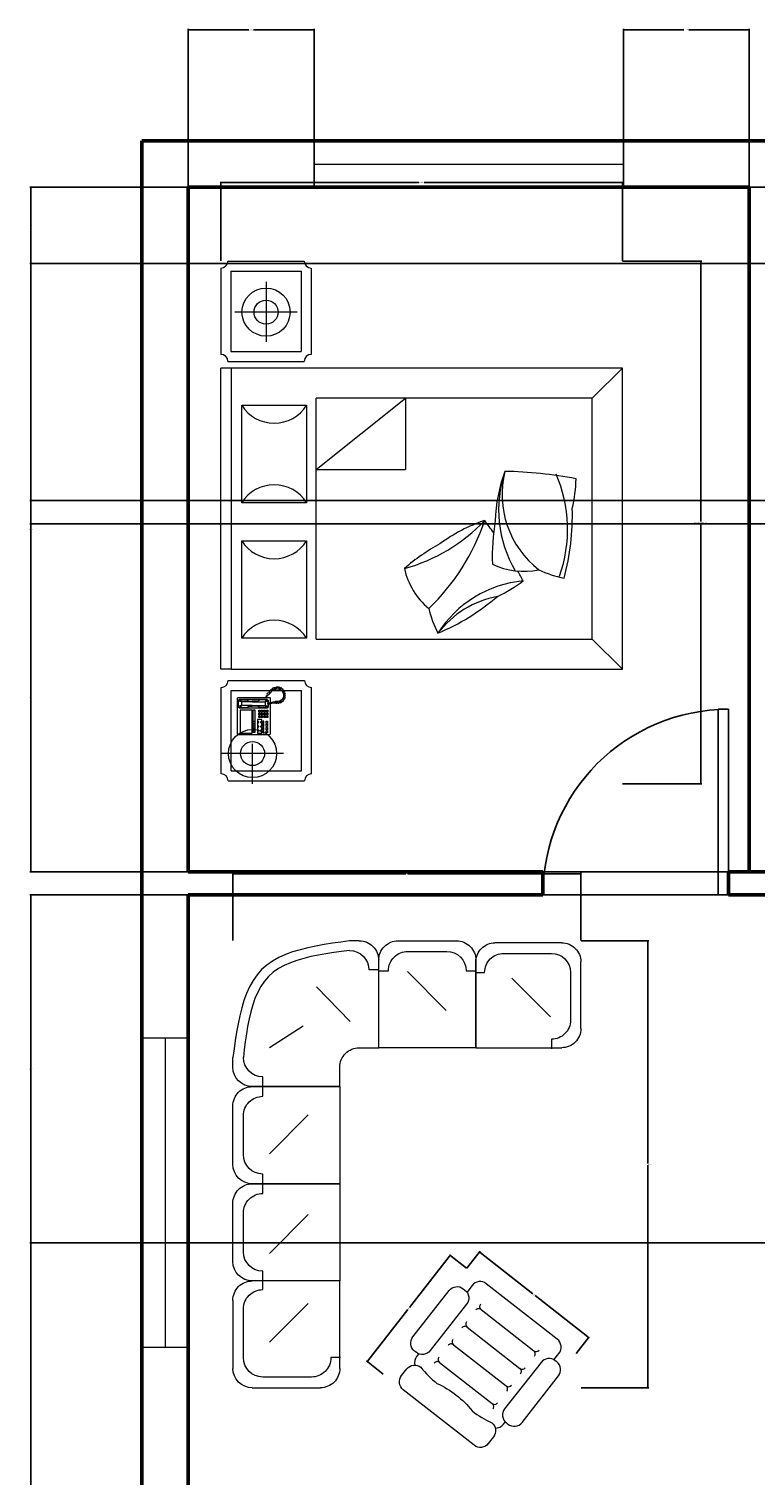
# Model space of a CAD drawing. Units: inches. Extents: x -108 to 1456, y -102 to 617.
# Tile 4 of 8: x 204 to 345, y 337 to 617. Entities that reach past the tile are written whole.
import ezdxf

# ---------------------------------------------------------------- set-up
doc = ezdxf.new("R2010")
doc.units = ezdxf.units.IN
for name, color, linetype, lineweight in [('A-ANNO-DIMS', 2, 'Continuous', 18), ('A-DOOR', 3, 'Continuous', 25), ('A-FURN', 8, 'Continuous', 18), ('A-GLAZ', 4, 'Continuous', 18), ('A-WALL', 7, 'Continuous', 50)]:
    doc.layers.add(name, color=color, linetype=linetype, lineweight=lineweight)
doc.styles.get("Standard").update_dxf_attribs({"font": 'arial.ttf'})
doc.dimstyles.get("Standard").update_dxf_attribs({"dimtxt": 0.18, "dimasz": 0.18, "dimexe": 0.18, "dimexo": 0.0625, "dimgap": 0.09, "dimtad": 0, "dimtih": 1, "dimtoh": 1, "dimdec": 4, "dimzin": 0, "dimdsep": 46, "dimtxsty": 'Standard', "dimcen": 0.09, "dimadec": 0, "dimazin": 0, "dimtfac": 1, "dimtdec": 4, "dimtofl": 0, "dimtmove": 0, "dimatfit": 3, "dimfxl": 1, "dimtolj": 1, "dimtzin": 0, "dimarcsym": 0})

# ---------------------------------------------------------------- blocks, each defined once
blk = doc.blocks.new('A$C50B66110')
for p, q in [((0.0153, 1.9631), (0.0153, 1.5831)), ((0.0503, 1.9981), (0.4803, 1.9981)), ((0.0653, 1.9481), (0.0653, 1.5981)), ((0.0653, 1.9481), (0.4653, 1.9481)), ((0.1513, 1.6871), (0.1513, 1.9967)), ((0.4653, 1.9481), (0.4653, 1.5981)), ((0.5153, 1.9631), (0.5153, 1.5831)), ((0.5716, 1.9488), (0.5716, 2)), ((0.5716, 2), (2.0719, 2)), ((2.0719, 1.9488), (0.5716, 1.9488)), ((0.5716, 1.9488), (0.5716, 0)), ((2.0719, 1.9488), (2.0719, 2)), ((2.0719, 0), (2.0719, 1.9488)), ((2.1051, 1.9643), (2.1051, 1.5843)), ((2.5701, 1.9993), (2.1401, 1.9993)), ((2.1551, 1.9493), (2.1551, 1.5993)), ((2.5551, 1.9493), (2.1551, 1.9493)), ((2.5551, 1.9493), (2.5551, 1.5993)), ((2.6051, 1.9643), (2.6051, 1.5843)), ((0.7257, 1.5725), (0.7257, 1.8954)), ((0.7257, 1.8954), (1.2113, 1.8954)), ((1.2113, 1.8954), (1.2113, 1.5725)), ((1.4007, 1.5725), (1.4007, 1.8954)), ((1.4007, 1.8954), (1.8863, 1.8954)), ((1.8863, 1.8954), (1.8863, 1.5725)), ((2.3505, 1.62), (2.3505, 1.9295)), ((0, 1.8416), (0.2001, 1.8416)), ((2.5018, 1.7744), (2.2017, 1.7744)), ((0.0653, 1.5981), (0.4653, 1.5981)), ((2.5551, 1.5993), (2.1551, 1.5993)), ((0.0503, 1.5481), (0.4803, 1.5481)), ((1.2113, 1.5725), (0.7257, 1.5725)), ((1.8863, 1.5725), (1.4007, 1.5725)), ((1.5665, 1.5254), (1.5665, 1.0802)), ((1.5665, 1.5254), (1.9219, 1.0802)), ((2.5701, 1.5493), (2.1401, 1.5493)), ((1.9219, 1.0802), (1.5665, 1.0802)), ((0.5716, 0), (0.7216, 0.15)), ((2.0719, 0), (1.9219, 0.15)), ((0.5716, 0), (2.0719, 0))]:
    blk.add_line(p, q)
at = {"linetype": 'ByBlock'}
for p, q in [((0.2481, 1.9162), (0.2458, 1.9139)), ((0.2458, 1.9139), (0.2458, 1.7562)), ((0.2481, 1.9162), (0.4287, 1.9162)), ((0.2526, 1.9036), (0.2526, 1.8431)), ((0.3669, 1.9036), (0.2526, 1.9036)), ((0.3669, 1.8431), (0.3669, 1.9036)), ((0.3772, 1.9071), (0.3818, 1.9128)), ((0.3772, 1.7688), (0.3772, 1.9071)), ((0.3818, 1.9094), (0.3807, 1.9048)), ((0.3807, 1.9048), (0.3807, 1.8739)), ((0.3807, 1.9048), (0.3909, 1.8945)), ((0.3807, 1.8739), (0.3829, 1.8682)), ((0.3818, 1.9128), (0.4161, 1.9128)), ((0.3864, 1.9116), (0.3818, 1.9094)), ((0.3921, 1.8968), (0.3864, 1.9116)), ((0.3864, 1.9116), (0.4138, 1.9116)), ((0.3909, 1.8945), (0.3921, 1.8968)), ((0.3909, 1.8431), (0.3909, 1.8945)), ((0.4081, 1.8968), (0.3921, 1.8968)), ((0.4081, 1.8968), (0.4138, 1.9116)), ((0.4092, 1.8945), (0.4081, 1.8968)), ((0.4195, 1.9048), (0.4092, 1.8945)), ((0.4092, 1.8431), (0.4092, 1.8945)), ((0.4138, 1.9116), (0.4184, 1.9094)), ((0.4161, 1.9128), (0.4218, 1.9071)), ((0.4195, 1.8739), (0.4172, 1.8682)), ((0.4184, 1.9094), (0.4195, 1.9048)), ((0.4195, 1.9048), (0.4195, 1.8739)), ((0.4218, 1.9071), (0.4218, 1.7699)), ((0.4287, 1.9162), (0.4309, 1.9139)), ((0.4309, 1.9139), (0.4309, 1.7562)), ((0.2526, 1.8431), (0.3669, 1.8431)), ((0.3201, 1.8168), (0.2526, 1.8168)), ((0.2526, 1.8168), (0.2526, 1.7962)), ((0.2572, 1.8408), (0.2572, 1.8294)), ((0.3669, 1.8408), (0.2572, 1.8408)), ((0.2572, 1.8294), (0.3669, 1.8294)), ((0.2675, 1.8145), (0.2641, 1.8145)), ((0.2641, 1.8145), (0.2641, 1.8111)), ((0.2641, 1.8111), (0.2675, 1.8111)), ((0.2641, 1.8019), (0.2641, 1.7985)), ((0.2675, 1.8019), (0.2641, 1.8019)), ((0.2664, 1.8408), (0.2664, 1.8294)), ((0.2675, 1.8111), (0.2675, 1.8145)), ((0.2675, 1.7985), (0.2675, 1.8019)), ((0.2755, 1.8408), (0.2755, 1.8294)), ((0.2846, 1.8408), (0.2846, 1.8294)), ((0.2846, 1.8145), (0.2846, 1.8111)), ((0.2881, 1.8145), (0.2846, 1.8145)), ((0.2846, 1.8111), (0.2881, 1.8111)), ((0.2846, 1.8019), (0.2846, 1.7985)), ((0.2881, 1.8019), (0.2846, 1.8019)), ((0.2881, 1.8111), (0.2881, 1.8145)), ((0.2881, 1.7985), (0.2881, 1.8019)), ((0.2938, 1.8408), (0.2938, 1.8294)), ((0.3029, 1.8408), (0.3029, 1.8294)), ((0.3052, 1.8145), (0.3052, 1.8111)), ((0.3086, 1.8145), (0.3052, 1.8145)), ((0.3052, 1.8111), (0.3086, 1.8111)), ((0.3052, 1.8019), (0.3052, 1.7985)), ((0.3086, 1.8019), (0.3052, 1.8019)), ((0.3086, 1.8111), (0.3086, 1.8145)), ((0.3086, 1.7985), (0.3086, 1.8019)), ((0.3121, 1.8408), (0.3121, 1.8294)), ((0.3201, 1.7962), (0.3201, 1.8168)), ((0.3304, 1.8111), (0.3395, 1.8111)), ((0.3304, 1.8042), (0.3304, 1.8111)), ((0.3395, 1.8042), (0.3304, 1.8042)), ((0.3395, 1.8111), (0.3395, 1.8042)), ((0.3441, 1.8042), (0.3441, 1.8111)), ((0.3441, 1.8111), (0.3532, 1.8111)), ((0.3532, 1.8042), (0.3441, 1.8042)), ((0.3532, 1.8111), (0.3532, 1.8042)), ((0.3578, 1.8111), (0.3669, 1.8111)), ((0.3578, 1.8042), (0.3578, 1.8111)), ((0.3669, 1.8042), (0.3578, 1.8042)), ((0.3669, 1.8294), (0.3669, 1.8408)), ((0.3669, 1.8111), (0.3669, 1.8042)), ((0.3807, 1.8019), (0.3829, 1.8076)), ((0.3807, 1.7711), (0.3807, 1.8019)), ((0.3829, 1.8682), (0.3864, 1.8625)), ((0.3829, 1.8076), (0.3864, 1.8134)), ((0.3864, 1.8625), (0.3875, 1.8545)), ((0.3864, 1.8134), (0.3875, 1.8214)), ((0.3875, 1.8545), (0.3875, 1.8431)), ((0.3875, 1.8214), (0.3875, 1.8431)), ((0.3909, 1.8431), (0.3909, 1.7813)), ((0.4092, 1.8431), (0.4092, 1.7813)), ((0.4138, 1.8625), (0.4127, 1.8545)), ((0.4127, 1.8545), (0.4127, 1.8431)), ((0.4127, 1.8214), (0.4127, 1.8431)), ((0.4138, 1.8134), (0.4127, 1.8214)), ((0.4172, 1.8682), (0.4138, 1.8625)), ((0.4172, 1.8076), (0.4138, 1.8134)), ((0.4195, 1.8019), (0.4172, 1.8076)), ((0.4195, 1.7711), (0.4195, 1.8019)), ((0.2458, 1.7562), (0.2481, 1.7539)), ((0.4, 1.7539), (0.2481, 1.7539)), ((0.2526, 1.7962), (0.3201, 1.7962)), ((0.2652, 1.7905), (0.2538, 1.7905)), ((0.2538, 1.7905), (0.2538, 1.7859)), ((0.2538, 1.7859), (0.2652, 1.7859)), ((0.2538, 1.7665), (0.2538, 1.7733)), ((0.2538, 1.7733), (0.2652, 1.7733)), ((0.2652, 1.7665), (0.2538, 1.7665)), ((0.2641, 1.7985), (0.2675, 1.7985)), ((0.2652, 1.7859), (0.2652, 1.7905)), ((0.2652, 1.7733), (0.2652, 1.7665)), ((0.2812, 1.7905), (0.2698, 1.7905)), ((0.2698, 1.7905), (0.2698, 1.7859)), ((0.2698, 1.7859), (0.2812, 1.7859)), ((0.2698, 1.7665), (0.2698, 1.7733)), ((0.2698, 1.7733), (0.2812, 1.7733)), ((0.2812, 1.7665), (0.2698, 1.7665)), ((0.2812, 1.7859), (0.2812, 1.7905)), ((0.2812, 1.7733), (0.2812, 1.7665)), ((0.2846, 1.7985), (0.2881, 1.7985)), ((0.2972, 1.7905), (0.2858, 1.7905)), ((0.2858, 1.7905), (0.2858, 1.7859)), ((0.2858, 1.7859), (0.2972, 1.7859)), ((0.2858, 1.7665), (0.2858, 1.7733)), ((0.2858, 1.7733), (0.2972, 1.7733)), ((0.2972, 1.7665), (0.2858, 1.7665)), ((0.2972, 1.7859), (0.2972, 1.7905)), ((0.2972, 1.7733), (0.2972, 1.7665)), ((0.3018, 1.7905), (0.3018, 1.7859)), ((0.3132, 1.7905), (0.3018, 1.7905)), ((0.3018, 1.7859), (0.3132, 1.7859)), ((0.3018, 1.7733), (0.3132, 1.7733)), ((0.3018, 1.7665), (0.3018, 1.7733)), ((0.3132, 1.7665), (0.3018, 1.7665)), ((0.3052, 1.7985), (0.3086, 1.7985)), ((0.3132, 1.7859), (0.3132, 1.7905)), ((0.3132, 1.7733), (0.3132, 1.7665)), ((0.3304, 1.7985), (0.3395, 1.7985)), ((0.3304, 1.7916), (0.3304, 1.7985)), ((0.3395, 1.7916), (0.3304, 1.7916)), ((0.3304, 1.7779), (0.3304, 1.7848)), ((0.3304, 1.7848), (0.3395, 1.7848)), ((0.3395, 1.7779), (0.3304, 1.7779)), ((0.3304, 1.7722), (0.3395, 1.7722)), ((0.3304, 1.7653), (0.3304, 1.7722)), ((0.3395, 1.7653), (0.3304, 1.7653)), ((0.3395, 1.7985), (0.3395, 1.7916)), ((0.3395, 1.7848), (0.3395, 1.7779)), ((0.3395, 1.7722), (0.3395, 1.7653)), ((0.3441, 1.7985), (0.3532, 1.7985)), ((0.3441, 1.7916), (0.3441, 1.7985)), ((0.3532, 1.7916), (0.3441, 1.7916)), ((0.3441, 1.7779), (0.3441, 1.7848)), ((0.3441, 1.7848), (0.3532, 1.7848)), ((0.3532, 1.7779), (0.3441, 1.7779)), ((0.3441, 1.7722), (0.3532, 1.7722)), ((0.3441, 1.7653), (0.3441, 1.7722)), ((0.3532, 1.7653), (0.3441, 1.7653)), ((0.3532, 1.7985), (0.3532, 1.7916)), ((0.3532, 1.7848), (0.3532, 1.7779)), ((0.3532, 1.7722), (0.3532, 1.7653)), ((0.3578, 1.7985), (0.3669, 1.7985)), ((0.3578, 1.7916), (0.3578, 1.7985)), ((0.3669, 1.7916), (0.3578, 1.7916)), ((0.3578, 1.7791), (0.3578, 1.7859)), ((0.3578, 1.7859), (0.3669, 1.7859)), ((0.3669, 1.7791), (0.3578, 1.7791)), ((0.3578, 1.7653), (0.3578, 1.7722)), ((0.3578, 1.7722), (0.3669, 1.7722)), ((0.3669, 1.7653), (0.3578, 1.7653)), ((0.3669, 1.7985), (0.3669, 1.7916)), ((0.3669, 1.7859), (0.3669, 1.7791)), ((0.3669, 1.7722), (0.3669, 1.7653)), ((0.3829, 1.7631), (0.3772, 1.7688)), ((0.3807, 1.7711), (0.3909, 1.7813)), ((0.3818, 1.7665), (0.3807, 1.7711)), ((0.3864, 1.7642), (0.3818, 1.7665)), ((0.399, 1.7631), (0.3829, 1.7631)), ((0.3921, 1.7791), (0.3864, 1.7642)), ((0.3864, 1.7642), (0.399, 1.7642)), ((0.3909, 1.7813), (0.3921, 1.7791)), ((0.4081, 1.7791), (0.3921, 1.7791)), ((0.4024, 1.7676), (0.3989, 1.7676)), ((0.3989, 1.7676), (0.3991, 1.7578)), ((0.3991, 1.7578), (0.4019, 1.7462)), ((0.4019, 1.7462), (0.4047, 1.7353)), ((0.403, 1.7585), (0.4024, 1.7676)), ((0.4026, 1.7642), (0.4138, 1.7642)), ((0.4161, 1.7631), (0.4027, 1.7631)), ((0.4047, 1.7511), (0.403, 1.7585)), ((0.4287, 1.7539), (0.404, 1.7539)), ((0.4047, 1.7353), (0.4044, 1.7293)), ((0.4044, 1.7293), (0.4051, 1.7279)), ((0.4074, 1.7402), (0.4047, 1.7511)), ((0.4081, 1.7346), (0.4074, 1.7402)), ((0.4079, 1.7286), (0.4081, 1.7346)), ((0.4092, 1.7813), (0.4081, 1.7791)), ((0.4081, 1.7791), (0.4138, 1.7642)), ((0.4195, 1.7711), (0.4092, 1.7813)), ((0.4138, 1.7642), (0.4184, 1.7665)), ((0.4218, 1.7699), (0.4161, 1.7631)), ((0.4184, 1.7665), (0.4195, 1.7711)), ((0.4309, 1.7562), (0.4287, 1.7539)), ((0.4378, 1.7742), (0.4309, 1.7768)), ((0.4309, 1.7722), (0.436, 1.7708)), ((0.436, 1.7708), (0.4406, 1.7672)), ((0.441, 1.771), (0.4378, 1.7742)), ((0.4406, 1.7672), (0.4418, 1.7656)), ((0.4434, 1.7688), (0.441, 1.771)), ((0.4443, 1.7658), (0.4418, 1.7633)), ((0.4418, 1.7656), (0.4443, 1.7658)), ((0.4418, 1.7633), (0.4511, 1.7551)), ((0.4477, 1.7704), (0.4434, 1.7688)), ((0.4497, 1.7684), (0.4477, 1.7704)), ((0.4481, 1.765), (0.4497, 1.7684)), ((0.4509, 1.7672), (0.4481, 1.765)), ((0.4539, 1.764), (0.4509, 1.7672)), ((0.4511, 1.7551), (0.4662, 1.7422)), ((0.4515, 1.7573), (0.4539, 1.764)), ((0.4577, 1.7605), (0.4515, 1.7573)), ((0.463, 1.7555), (0.4577, 1.7605)), ((0.4618, 1.7482), (0.463, 1.7555)), ((0.467, 1.7515), (0.4618, 1.7482)), ((0.4664, 1.7418), (0.4741, 1.72)), ((0.4714, 1.7468), (0.467, 1.7515)), ((0.4696, 1.7418), (0.4714, 1.7468)), ((0.4766, 1.7425), (0.4697, 1.7418)), ((0.472, 1.733), (0.4787, 1.7356)), ((0.4794, 1.7332), (0.472, 1.733)), ((0.4787, 1.7356), (0.4766, 1.7425)), ((0.481, 1.7279), (0.4794, 1.7332)), ((0.4026, 1.7254), (0.4021, 1.7198)), ((0.4021, 1.7198), (0.4088, 1.7187)), ((0.4088, 1.7187), (0.4023, 1.7147)), ((0.4023, 1.7147), (0.4028, 1.7085)), ((0.4051, 1.7279), (0.4026, 1.7254)), ((0.4028, 1.7085), (0.4102, 1.7078)), ((0.4102, 1.7078), (0.4037, 1.7027)), ((0.4037, 1.7027), (0.4067, 1.6974)), ((0.4067, 1.6974), (0.4137, 1.6988)), ((0.4121, 1.7256), (0.4079, 1.7286)), ((0.4137, 1.6988), (0.4104, 1.6923)), ((0.4104, 1.6923), (0.4139, 1.6881)), ((0.4111, 1.7203), (0.4121, 1.7256)), ((0.4123, 1.7057), (0.4111, 1.7203)), ((0.4211, 1.6946), (0.4123, 1.7057)), ((0.4139, 1.6881), (0.4192, 1.692)), ((0.4192, 1.692), (0.4183, 1.6858)), ((0.4183, 1.6858), (0.4227, 1.683)), ((0.4333, 1.6881), (0.4211, 1.6946)), ((0.4227, 1.683), (0.4283, 1.6876)), ((0.4283, 1.6876), (0.4276, 1.68)), ((0.4276, 1.68), (0.4324, 1.6786)), ((0.4324, 1.6786), (0.4354, 1.6849)), ((0.4472, 1.6869), (0.4333, 1.6881)), ((0.4354, 1.6849), (0.4382, 1.6786)), ((0.4382, 1.6786), (0.4421, 1.6782)), ((0.4421, 1.6782), (0.4437, 1.6849)), ((0.4437, 1.6849), (0.4463, 1.6775)), ((0.4463, 1.6775), (0.4507, 1.6786)), ((0.4606, 1.6927), (0.4472, 1.6869)), ((0.4507, 1.6786), (0.4509, 1.6849)), ((0.4509, 1.6849), (0.4562, 1.6802)), ((0.4562, 1.6802), (0.4599, 1.6821)), ((0.4592, 1.689), (0.4641, 1.683)), ((0.4599, 1.6821), (0.4592, 1.689)), ((0.4708, 1.7027), (0.4606, 1.6927)), ((0.4641, 1.683), (0.4678, 1.6863)), ((0.465, 1.6925), (0.4715, 1.6897)), ((0.4678, 1.6863), (0.465, 1.6925)), ((0.4741, 1.72), (0.4708, 1.7027)), ((0.4745, 1.6925), (0.4713, 1.6988)), ((0.4713, 1.6988), (0.478, 1.6967)), ((0.4715, 1.6897), (0.4745, 1.6925)), ((0.4743, 1.7075), (0.4815, 1.7073)), ((0.4798, 1.7013), (0.4743, 1.7075)), ((0.4761, 1.7233), (0.481, 1.7279)), ((0.4824, 1.7233), (0.4761, 1.7233)), ((0.4764, 1.7154), (0.4835, 1.7175)), ((0.4824, 1.7119), (0.4764, 1.7154)), ((0.478, 1.6967), (0.4798, 1.7013)), ((0.4815, 1.7073), (0.4824, 1.7119)), ((0.4835, 1.7175), (0.4824, 1.7233)), ((0.7216, 1.5254), (1.9219, 1.5254)), ((0.7216, 1.5254), (0.7216, 0.15)), ((1.9219, 0.15), (1.9219, 1.5254)), ((0.7216, 0.15), (1.9219, 0.15))]:
    blk.add_line(p, q, dxfattribs=at)
for centre, radius in [((0.1513, 1.8416), 0.12), ((0.1513, 1.8416), 0.06), ((2.3505, 1.7744), 0.12), ((2.3505, 1.7744), 0.06)]:
    blk.add_circle(centre, radius)
for centre, radius, start, end in [((0.0153, 1.9981), 0.035, 270, 0), ((0.5153, 1.9981), 0.035, 180, 270), ((2.1051, 1.9993), 0.035, 270, 0), ((2.6051, 1.9993), 0.035, 180, 270), ((0.6244, 1.734), 0.1906, 302.12017, 57.87983), ((1.3126, 1.734), 0.1906, 122.12017, 237.87983), ((1.2994, 1.734), 0.1906, 302.12017, 57.87983), ((1.9876, 1.734), 0.1906, 122.12017, 237.87983), ((0.0153, 1.5481), 0.035, 0, 90), ((0.5153, 1.5481), 0.035, 90, 180), ((2.1051, 1.5493), 0.035, 0, 90), ((2.6051, 1.5493), 0.035, 90, 180), ((1.1502, 0.7366), 0.3575, 102.47819, 140.46254), ((0.328, 0.4368), 0.9879, 28.49711, 41.05657), ((1.9117, 1.3157), 0.8697, 195.33601, 226.41927), ((0.9996, 0.4307), 0.548, 103.20343, 117.03623), ((1.656, 1.7093), 1.0798, 223.63057, 251.4288), ((0.4482, 0.4408), 0.5655, 5.33912, 57.68949), ((1.8226, 1.3753), 1.1652, 203.06416, 220.32086), ((0.4548, 0.5307), 0.4879, 10.69865, 52.68638), ((0.5648, 0.4378), 0.7874, 18.35266, 36.68512), ((-0.0179, 2.4352), 2.1977, 305.29657, 307.24182), ((1.5981, 0.9345), 0.734, 205.25901, 216.93514), ((1.4166, 0.4903), 0.3575, 154.0418, 192.02615), ((1.3672, 0.0075), 0.6085, 71.81005, 120.13512), ((1.4431, 0.1219), 0.4774, 76.18494, 142.00166), ((1.1403, -0.3401), 0.9879, 80.06073, 92.62018), ((1.2867, -0.154), 0.7874, 69.91627, 88.24873), ((-0.6401, 0.6314), 2.1977, 349.48843, 358.80544), ((-0.0179, 2.4352), 2.1977, 297.92482, 299.3793), ((1.5626, 0.1822), 0.548, 154.76704, 168.59984), ((1.3343, 1.4141), 1.1652, 254.62778, 271.88448), ((1.2678, 0.9611), 0.6885, 250.29361, 293.6414), ((1.5399, 0.9642), 0.734, 256.82263, 268.49876)]:
    blk.add_arc(centre, radius, start, end)
blk = doc.blocks.new('A$C4B324E0D')
for points in [[(-0.4032, -0.0374), (-0.3959, 0.0153), (-0.3883, 0.0678), (-0.3801, 0.1195), (-0.3709, 0.1704), (-0.3605, 0.22), (-0.3485, 0.2679), (-0.3346, 0.314), (-0.3185, 0.3579), (-0.2998, 0.3993), (-0.2783, 0.4378), (-0.2537, 0.4731), (-0.2255, 0.5049), (-0.1936, 0.5331), (-0.1583, 0.5578), (-0.1198, 0.5793), (-0.0785, 0.5979), (-0.0346, 0.614), (0.0115, 0.628), (0.0595, 0.64), (0.1091, 0.6504), (0.1599, 0.6595), (0.2117, 0.6678), (0.2641, 0.6753), (0.3168, 0.6826)], [(0.3768, 0.6826), (0.3168, 0.6826)], [(0.9768, 0.6826), (0.6168, 0.6826)], [(1.5769, 0.6826), (1.2168, 0.6826)], [(1.8168, 0.6826), (2.2368, 0.6826)], [(-0.3432, -0.0374), (-0.3369, 0.0114), (-0.3303, 0.0599), (-0.3232, 0.1078), (-0.3151, 0.1548), (-0.3059, 0.2006), (-0.2951, 0.2449), (-0.2826, 0.2874), (-0.2681, 0.3278), (-0.2511, 0.3658), (-0.2315, 0.4011), (-0.2089, 0.4335), (-0.1831, 0.4625), (-0.1538, 0.488), (-0.1214, 0.5102), (-0.086, 0.5294), (-0.0479, 0.546), (-0.0075, 0.5602), (0.035, 0.5722), (0.0793, 0.5825), (0.125, 0.5914), (0.172, 0.599), (0.2198, 0.6057), (0.2682, 0.6119), (0.3168, 0.6177)], [(0.3168, 0.6177), (0.3168, 0.6177)], [(0.4968, 0.0226), (0.4968, 0.5626)], [(0.4968, 0.5626), (0.4968, 0.0226), (1.0968, 0.0226)], [(0.9168, 0.6177), (0.6768, 0.6177)], [(1.0968, 0.5626), (1.0968, 0.0226), (1.6968, 0.0226)], [(1.0968, 0.0226), (1.0968, 0.5626)], [(1.5168, 0.6177), (1.2768, 0.6177)], [(1.6968, 0.0226), (1.6968, 0.5626)], [(2.2368, 0.0226), (1.6968, 0.0226), (1.6968, 0.5626)], [(2.1704, 0.6177), (1.8704, 0.6177)], [(2.3569, 0.5626), (2.3569, 0.1426)], [(0.255, 0.4573), (0.1211, 0.2495)], [(0.4968, 0.4977), (0.4368, 0.4977), (0.4368, 0.4977)], [(0.5569, 0.4977), (0.5569, 0.4977), (0.4968, 0.4977)], [(0.9111, 0.4573), (0.6711, 0.2173)], [(1.0968, 0.4977), (1.0368, 0.4977), (1.0368, 0.4977)], [(1.1569, 0.4977), (1.1569, 0.4977), (1.0968, 0.4977)], [(1.527, 0.4573), (1.287, 0.2173)], [(1.6969, 0.4977), (1.6368, 0.4977), (1.6368, 0.4977)], [(1.7504, 0.4977), (1.7504, 0.4977), (1.6904, 0.4977)], [(2.0759, 0.4573), (1.8359, 0.2173)], [(2.2904, 0.1977), (2.2904, 0.4977)], [(-0.1199, 0.1664), (0.0943, -0.0414)], [(0.4968, 0.0226), (0.3768, 0.0226)], [(2.1704, 0.0177), (2.1704, 0.0777), (2.1704, 0.0777)], [(-0.4032, -0.0974), (-0.4032, -0.0374)], [(-0.3432, -0.0374), (-0.3432, -0.0374)], [(-0.2232, -0.2174), (-0.2232, -0.1574), (-0.2232, -0.1574)], [(0.2568, -0.0974), (0.2568, -0.2174)], [(-0.2832, -0.8174), (0.2568, -0.8174), (0.2568, -0.2174)], [(0.2568, -0.2174), (-0.2832, -0.2174)], [(0.2568, -0.2174), (-0.2832, -0.2174)], [(-0.2183, -0.2174), (-0.2183, -0.2774), (-0.2183, -0.2774)], [(-0.4032, -0.3374), (-0.4032, -0.6974)], [(-0.3383, -0.3974), (-0.3383, -0.6374)], [(-0.2136, -0.3946), (0.0264, -0.6346)], [(-0.2183, -0.7574), (-0.2183, -0.7574), (-0.2183, -0.8174)], [(0.2568, -0.8174), (-0.2832, -0.8174)], [(-0.2732, -0.8174), (0.2568, -0.8174), (0.2568, -1.3475)], [(-0.208, -0.8126), (-0.208, -0.8715), (-0.208, -0.8715)], [(0.2568, -0.8174), (0.2568, -1.3475)], [(-0.391, -1.3475), (-0.391, -0.9352)], [(-0.3258, -0.9893), (-0.3258, -1.2838)], [(-0.1734, -1.0387), (0.0666, -1.2787)], [(0.2043, -1.2838), (0.2043, -1.2838), (0.2632, -1.2838)], [(-0.208, -1.4016), (0.0865, -1.4016)], [(0.1391, -1.4653), (-0.2732, -1.4653)]]:
    blk.add_lwpolyline(points)
for centre, radius, start, end in [((0.3768, 0.5626), 0.12, 0, 90), ((0.6168, 0.5626), 0.12, 90, 180), ((0.9768, 0.5626), 0.12, 0, 90), ((1.2168, 0.5626), 0.12, 90, 180), ((1.5769, 0.5626), 0.12, 0, 90), ((1.8168, 0.5626), 0.12, 90, 180), ((2.2368, 0.5626), 0.12, 0, 90), ((0.3168, 0.4977), 0.12, 0, 90), ((0.6768, 0.4977), 0.12, 90, 180), ((0.9168, 0.4977), 0.12, 0, 90), ((1.2768, 0.4977), 0.12, 90, 180), ((1.5168, 0.4977), 0.12, 0, 90), ((1.8704, 0.4977), 0.12, 90, 180), ((2.1704, 0.4977), 0.12, 0, 90), ((2.1704, 0.1977), 0.12, 270, 0), ((2.2368, 0.1426), 0.12, 270, 0), ((0.3768, -0.0974), 0.12, 90, 180), ((-0.2232, -0.0374), 0.12, 180, 270), ((-0.2832, -0.0974), 0.12, 179.9997, 270), ((-0.2832, -0.3374), 0.12, 90, 180), ((-0.2183, -0.3974), 0.12, 90, 180), ((-0.2832, -0.6974), 0.12, 179.9997, 270), ((-0.2183, -0.6374), 0.12, 180, 270), ((-0.2732, -0.9352), 0.1178, 90, 180), ((-0.208, -0.9893), 0.1178, 90, 180), ((-0.208, -1.2838), 0.1178, 180, 270), ((0.0865, -1.2838), 0.1178, 270, 0), ((-0.2732, -1.3475), 0.1178, 179.9997, 270), ((0.1391, -1.3475), 0.1178, 270, 0)]:
    blk.add_arc(centre, radius, start, end)
blk = doc.blocks.new('A$C58C6152E')
at = {"xscale": 1.5, "yscale": 1.5, "zscale": 1.5, "rotation": 90}
blk.add_blockref('A$C4B324E0D', (1.024, 0.605), dxfattribs=at)
blk = doc.blocks.new('A$C15DC316E')
at = {"xscale": -1, "rotation": 270}
blk.add_blockref('A$C58C6152E', (0, 0), dxfattribs=at)
blk = doc.blocks.new('A$C31080000')
for p, q in [((364.2, 324.1), (125.4, 324.1)), ((364.2, 244.1), (125.4, 244.1)), ((364.2, 164.1), (125.4, 164.1)), ((364.2, 84.1), (125.4, 84.1)), ((442.3, 35.8), (442.3, 67.5))]:
    blk.add_line(p, q)
for points in [[(48.5, 445.3, -0.414214), (84.3, 481.1), (406.4, 481.1, -0.414214), (442.2, 445.3), (442.2, 415.1, -0.414214), (406.4, 379.4)], [(406.4, 379.4, 0.055299), (325.4, 388.9, -0.118462), (165.4, 388.9, 0.055299), (84.3, 379.4, -0.414214), (48.5, 415.1), (48.5, 445.3, -0.414214)], [(62.9, 386.5, 0.236068), (48.5, 357.9), (48.5, 347.9)], [(442.2, 345.6), (442.2, 357.9, 0.236068), (427.9, 386.5)], [(48.5, 65.5), (48.5, 35.8, 0.414214), (84.3, 0), (406.4, 0, 0.414214), (442.2, 35.8)]]:
    blk.add_lwpolyline(points, format="xyb")
for points in [[(78.9, 311.7, 0.414214), (43.1, 347.5), (35.8, 347.5, 0.414214), (0, 311.7), (0, 100.6, 0.414214), (35.8, 64.8), (43.1, 64.8, 0.414214), (78.9, 100.6)], [(416.7, 311.7, -0.414214), (452.5, 347.5), (459.8, 347.5, -0.414214), (495.6, 311.7), (495.6, 100.6, -0.414214), (459.8, 64.8), (452.5, 64.8, -0.414214), (416.7, 100.6)]]:
    blk.add_lwpolyline(points, format="xyb", close=True)
for centre, start, end in [((125.4, 337.6), 180, 270), ((125.4, 310.5), 90, 180), ((364.2, 337.6), 270, 0), ((364.2, 310.5), 0, 90), ((125.4, 257.6), 180, 270), ((125.4, 230.5), 90, 180), ((364.2, 257.6), 270, 0), ((364.2, 230.5), 0, 90), ((125.4, 177.6), 180, 270), ((125.4, 150.5), 90, 180), ((364.2, 177.6), 270, 0), ((364.2, 150.5), 0, 90), ((125.4, 97.6), 180, 270), ((125.4, 70.5), 90, 180), ((364.2, 97.6), 270, 0), ((364.2, 70.5), 0, 90)]:
    blk.add_arc(centre, 13.6, start, end)
blk = doc.blocks.new('DOOR-36-SWING')
for p, q in [((36, 36), (34, 36)), ((34, 36), (34, 0)), ((36, 36), (34, 36)), ((36, 0), (36, 36)), ((34, 0), (36, 0))]:
    blk.add_line(p, q)
blk.add_arc((36, 36), 36, 180, 270)
blk = doc.blocks.new('WIN-60-WALL-9')
for p, q in [((0, 0), (0, 9)), ((60, 0), (60, 9)), ((0, 4.5), (60, 4.5))]:
    blk.add_line(p, q)
blk = doc.blocks.new('*D20')
at = {"layer": 'A-ANNO-DIMS', "color": 0, "lineweight": -2, "transparency": 16777216}
for p, q in [((319.55, 572.46), (334.88, 572.46)), ((334.7, 572.28), (334.7, 521.94)), ((334.7, 471.23), (334.7, 521.57)), ((319.55, 471.05), (334.88, 471.05))]:
    blk.add_line(p, q, dxfattribs=at)
at = {"layer": 'A-ANNO-DIMS', "color": 0, "transparency": 16777216}
for points in [[(334.67, 572.28), (334.73, 572.28), (334.7, 572.46)], [(334.67, 471.23), (334.73, 471.23), (334.7, 471.05)]]:
    blk.add_solid(points, dxfattribs=at)
at = {"layer": 'Defpoints', "color": 0, "transparency": 16777216}
for p in [(319.49, 572.46), (334.7, 572.46), (319.49, 471.05)]:
    blk.add_point(p, dxfattribs=at)
at = {"layer": 'A-ANNO-DIMS', "color": 0, "transparency": 16777216, "insert": (334.7, 521.75), "char_height": 0.18, "attachment_point": 5}
blk.add_mtext('\\A1;BED GROUP 101 TYP.', dxfattribs=at)
blk = doc.blocks.new('*D21')
at = {"layer": 'A-ANNO-DIMS', "color": 0, "lineweight": -2, "transparency": 16777216}
for p, q in [((241.63, 572.52), (241.63, 587.85)), ((241.81, 587.67), (280.03, 587.67)), ((319.31, 587.67), (281.09, 587.67)), ((319.49, 572.52), (319.49, 587.85))]:
    blk.add_line(p, q, dxfattribs=at)
at = {"layer": 'A-ANNO-DIMS', "color": 0, "transparency": 16777216}
for points in [[(241.81, 587.7), (241.81, 587.64), (241.63, 587.67)], [(319.31, 587.7), (319.31, 587.64), (319.49, 587.67)]]:
    blk.add_solid(points, dxfattribs=at)
at = {"layer": 'Defpoints', "color": 0, "transparency": 16777216}
for p in [(241.63, 587.67), (241.63, 572.46), (319.49, 572.46)]:
    blk.add_point(p, dxfattribs=at)
at = {"layer": 'A-ANNO-DIMS', "color": 0, "transparency": 16777216, "insert": (280.56, 587.67), "char_height": 0.18, "attachment_point": 5}
blk.add_mtext('\\A1;78 TYP.', dxfattribs=at)
blk = doc.blocks.new('*D30')
at = {"layer": 'A-ANNO-DIMS', "color": 0, "lineweight": -2, "transparency": 16777216}
for p, q in [((311.51, 440.62), (324.63, 440.62)), ((324.45, 440.44), (324.45, 397.46)), ((324.45, 354.11), (324.45, 397.09)), ((311.51, 353.93), (324.63, 353.93))]:
    blk.add_line(p, q, dxfattribs=at)
at = {"layer": 'A-ANNO-DIMS', "color": 0, "transparency": 16777216}
for points in [[(324.42, 440.44), (324.48, 440.44), (324.45, 440.62)], [(324.42, 354.11), (324.48, 354.11), (324.45, 353.93)]]:
    blk.add_solid(points, dxfattribs=at)
at = {"layer": 'Defpoints', "color": 0, "transparency": 16777216}
for p in [(311.44, 440.62), (311.44, 353.93), (324.45, 353.93)]:
    blk.add_point(p, dxfattribs=at)
at = {"layer": 'A-ANNO-DIMS', "color": 0, "transparency": 16777216, "insert": (324.45, 397.27), "char_height": 0.18, "attachment_point": 5}
blk.add_mtext('\\A1;SECTIONAL 87', dxfattribs=at)
blk = doc.blocks.new('*D31')
at = {"layer": 'A-ANNO-DIMS', "color": 0, "lineweight": -2, "transparency": 16777216}
for p, q in [((243.98, 440.68), (243.98, 453.8)), ((244.16, 453.62), (277.49, 453.62)), ((311.26, 453.62), (277.93, 453.62)), ((311.44, 440.68), (311.44, 453.8))]:
    blk.add_line(p, q, dxfattribs=at)
at = {"layer": 'A-ANNO-DIMS', "color": 0, "transparency": 16777216}
for points in [[(244.16, 453.65), (244.16, 453.59), (243.98, 453.62)], [(311.26, 453.65), (311.26, 453.59), (311.44, 453.62)]]:
    blk.add_solid(points, dxfattribs=at)
at = {"layer": 'Defpoints', "color": 0, "transparency": 16777216}
for p in [(311.44, 453.62), (243.98, 440.62), (311.44, 440.62)]:
    blk.add_point(p, dxfattribs=at)
at = {"layer": 'A-ANNO-DIMS', "color": 0, "transparency": 16777216, "insert": (277.71, 453.62), "char_height": 0.18, "attachment_point": 5}
blk.add_mtext('\\A1;67', dxfattribs=at)
blk = doc.blocks.new('*D32')
at = {"layer": 'A-ANNO-DIMS', "color": 0, "lineweight": -2, "transparency": 16777216}
for p, q in [((289.34, 377.15), (291.9, 380.42)), ((291.93, 380.17), (302.14, 372.17)), ((312.83, 363.8), (302.61, 371.8)), ((310.52, 360.56), (313.08, 363.83))]:
    blk.add_line(p, q, dxfattribs=at)
at = {"layer": 'A-ANNO-DIMS', "color": 0, "transparency": 16777216}
for points in [[(291.95, 380.19), (291.91, 380.14), (291.79, 380.28)], [(312.84, 363.83), (312.81, 363.78), (312.97, 363.69)]]:
    blk.add_solid(points, dxfattribs=at)
at = {"layer": 'Defpoints', "color": 0, "transparency": 16777216}
for p in [(291.79, 380.28), (289.3, 377.1), (310.48, 360.51)]:
    blk.add_point(p, dxfattribs=at)
at = {"layer": 'A-ANNO-DIMS', "color": 0, "transparency": 16777216, "insert": (302.38, 371.98), "char_height": 0.18, "attachment_point": 5}
blk.add_mtext('\\A1;CHAIR 27', dxfattribs=at)
blk = doc.blocks.new('*D33')
at = {"layer": 'A-ANNO-DIMS', "color": 0, "lineweight": -2, "transparency": 16777216}
for p, q in [((286.01, 379.45), (278.21, 369.49)), ((289.25, 377.14), (285.98, 379.7)), ((270.13, 359.17), (277.93, 369.13)), ((273.15, 356.58), (269.88, 359.14))]:
    blk.add_line(p, q, dxfattribs=at)
at = {"layer": 'A-ANNO-DIMS', "color": 0, "transparency": 16777216}
for points in [[(285.99, 379.47), (286.03, 379.43), (286.12, 379.59)], [(270.1, 359.19), (270.15, 359.15), (270.02, 359.03)]]:
    blk.add_solid(points, dxfattribs=at)
at = {"layer": 'Defpoints', "color": 0, "transparency": 16777216}
for p in [(289.3, 377.1), (270.02, 359.03), (273.19, 356.54)]:
    blk.add_point(p, dxfattribs=at)
at = {"layer": 'A-ANNO-DIMS', "color": 0, "transparency": 16777216, "insert": (278.07, 369.31), "char_height": 0.18, "attachment_point": 5}
blk.add_mtext('\\A1;26', dxfattribs=at)
blk = doc.blocks.new('*D36')
at = {"layer": 'A-ANNO-DIMS', "color": 0, "lineweight": -2, "transparency": 16777216}
for p, q in [((235.34, 586.84), (235.34, 617.48)), ((235.52, 617.3), (247.07, 617.3)), ((259.54, 617.3), (248, 617.3)), ((259.72, 586.84), (259.72, 617.48))]:
    blk.add_line(p, q, dxfattribs=at)
at = {"layer": 'A-ANNO-DIMS', "color": 0, "transparency": 16777216}
for points in [[(235.52, 617.33), (235.52, 617.27), (235.34, 617.3)], [(259.54, 617.33), (259.54, 617.27), (259.72, 617.3)]]:
    blk.add_solid(points, dxfattribs=at)
at = {"layer": 'Defpoints', "color": 0, "transparency": 16777216}
for p in [(259.72, 617.3), (235.34, 586.77), (259.72, 586.77)]:
    blk.add_point(p, dxfattribs=at)
at = {"layer": 'A-ANNO-DIMS', "color": 0, "transparency": 16777216, "insert": (247.53, 617.3), "char_height": 0.18, "attachment_point": 5}
blk.add_mtext('\\A1;24.375', dxfattribs=at)
blk = doc.blocks.new('*D37')
at = {"layer": 'A-ANNO-DIMS', "color": 0, "lineweight": -2, "transparency": 16777216}
for p, q in [((319.72, 586.84), (319.72, 617.48)), ((319.9, 617.3), (331.44, 617.3)), ((343.91, 617.3), (332.37, 617.3)), ((344.09, 586.84), (344.09, 617.48))]:
    blk.add_line(p, q, dxfattribs=at)
at = {"layer": 'A-ANNO-DIMS', "color": 0, "transparency": 16777216}
for points in [[(319.9, 617.33), (319.9, 617.27), (319.72, 617.3)], [(343.91, 617.33), (343.91, 617.27), (344.09, 617.3)]]:
    blk.add_solid(points, dxfattribs=at)
at = {"layer": 'Defpoints', "color": 0, "transparency": 16777216}
for p in [(344.09, 617.3), (319.72, 586.77), (344.09, 586.77)]:
    blk.add_point(p, dxfattribs=at)
at = {"layer": 'A-ANNO-DIMS', "color": 0, "transparency": 16777216, "insert": (331.91, 617.3), "char_height": 0.18, "attachment_point": 5}
blk.add_mtext('\\A1;24.375', dxfattribs=at)
blk = doc.blocks.new('*D39')
at = {"layer": 'A-ANNO-DIMS', "color": 0, "lineweight": -2, "transparency": 16777216}
for p, q in [((235.28, 586.77), (204.64, 586.77)), ((204.82, 586.59), (204.82, 520.58)), ((204.82, 454.2), (204.82, 520.22)), ((235.28, 454.02), (204.64, 454.02))]:
    blk.add_line(p, q, dxfattribs=at)
at = {"layer": 'A-ANNO-DIMS', "color": 0, "transparency": 16777216}
for points in [[(204.79, 586.59), (204.85, 586.59), (204.82, 586.77)], [(204.79, 454.2), (204.85, 454.2), (204.82, 454.02)]]:
    blk.add_solid(points, dxfattribs=at)
at = {"layer": 'Defpoints', "color": 0, "transparency": 16777216}
for p in [(235.34, 586.77), (204.82, 454.02), (235.34, 454.02)]:
    blk.add_point(p, dxfattribs=at)
at = {"layer": 'A-ANNO-DIMS', "color": 0, "transparency": 16777216, "insert": (204.82, 520.4), "char_height": 0.18, "attachment_point": 5}
blk.add_mtext('\\A1;132.75', dxfattribs=at)
blk = doc.blocks.new('*D40')
at = {"layer": 'A-ANNO-DIMS', "color": 0, "lineweight": -2, "transparency": 16777216}
for p, q in [((235.28, 449.52), (204.64, 449.52)), ((204.82, 449.34), (204.82, 391.96)), ((204.82, 334.2), (204.82, 391.59)), ((235.28, 334.02), (204.64, 334.02))]:
    blk.add_line(p, q, dxfattribs=at)
at = {"layer": 'A-ANNO-DIMS', "color": 0, "transparency": 16777216}
for points in [[(204.79, 449.34), (204.85, 449.34), (204.82, 449.52)], [(204.79, 334.2), (204.85, 334.2), (204.82, 334.02)]]:
    blk.add_solid(points, dxfattribs=at)
at = {"layer": 'Defpoints', "color": 0, "transparency": 16777216}
for p in [(235.34, 449.52), (204.82, 334.02), (235.34, 334.02)]:
    blk.add_point(p, dxfattribs=at)
at = {"layer": 'A-ANNO-DIMS', "color": 0, "transparency": 16777216, "insert": (204.82, 391.77), "char_height": 0.18, "attachment_point": 5}
blk.add_mtext('\\A1;115.5', dxfattribs=at)
blk = doc.blocks.new('*D45')
at = {"layer": 'A-ANNO-DIMS', "color": 0, "lineweight": -2, "transparency": 16777216}
for p, q in [((348.2, 521.52), (204.64, 521.52)), ((204.82, 521.34), (204.82, 487.96)), ((204.82, 454.2), (204.82, 487.59)), ((348.2, 454.02), (204.64, 454.02))]:
    blk.add_line(p, q, dxfattribs=at)
at = {"layer": 'A-ANNO-DIMS', "color": 0, "transparency": 16777216}
for points in [[(204.79, 521.34), (204.85, 521.34), (204.82, 521.52)], [(204.79, 454.2), (204.85, 454.2), (204.82, 454.02)]]:
    blk.add_solid(points, dxfattribs=at)
at = {"layer": 'Defpoints', "color": 0, "transparency": 16777216}
for p in [(204.82, 521.52), (348.27, 521.52), (348.27, 454.02)]:
    blk.add_point(p, dxfattribs=at)
at = {"layer": 'A-ANNO-DIMS', "color": 0, "transparency": 16777216, "insert": (204.82, 487.77), "char_height": 0.18, "attachment_point": 5}
blk.add_mtext('\\A1;67.5', dxfattribs=at)
blk = doc.blocks.new('*D46')
at = {"layer": 'A-ANNO-DIMS', "color": 0, "lineweight": -2, "transparency": 16777216}
for p, q in [((348.2, 526.02), (204.64, 526.02)), ((204.82, 525.84), (204.82, 523.96)), ((204.82, 521.7), (204.82, 523.59)), ((348.2, 521.52), (204.64, 521.52))]:
    blk.add_line(p, q, dxfattribs=at)
at = {"layer": 'A-ANNO-DIMS', "color": 0, "transparency": 16777216}
for points in [[(204.79, 525.84), (204.85, 525.84), (204.82, 526.02)], [(204.79, 521.7), (204.85, 521.7), (204.82, 521.52)]]:
    blk.add_solid(points, dxfattribs=at)
at = {"layer": 'Defpoints', "color": 0, "transparency": 16777216}
for p in [(348.27, 526.02), (204.82, 521.52), (348.27, 521.52)]:
    blk.add_point(p, dxfattribs=at)
at = {"layer": 'A-ANNO-DIMS', "color": 0, "transparency": 16777216, "insert": (204.82, 523.77), "char_height": 0.18, "attachment_point": 5}
blk.add_mtext('\\A1;4.5', dxfattribs=at)
blk = doc.blocks.new('*D51')
at = {"layer": 'A-ANNO-DIMS', "color": 0, "lineweight": -2, "transparency": 16777216}
for p, q in [((348.53, 586.77), (204.64, 586.77)), ((204.82, 586.59), (204.82, 579.56)), ((204.82, 572.16), (204.82, 579.2)), ((348.89, 571.98), (204.64, 571.98))]:
    blk.add_line(p, q, dxfattribs=at)
at = {"layer": 'A-ANNO-DIMS', "color": 0, "transparency": 16777216}
for points in [[(204.79, 586.59), (204.85, 586.59), (204.82, 586.77)], [(204.79, 572.16), (204.85, 572.16), (204.82, 571.98)]]:
    blk.add_solid(points, dxfattribs=at)
at = {"layer": 'Defpoints', "color": 0, "transparency": 16777216}
for p in [(348.59, 586.77), (204.82, 571.98), (348.95, 571.98)]:
    blk.add_point(p, dxfattribs=at)
at = {"layer": 'A-ANNO-DIMS', "color": 0, "transparency": 16777216, "insert": (204.82, 579.38), "char_height": 0.18, "attachment_point": 5}
blk.add_mtext('\\A1;14.79', dxfattribs=at)
blk = doc.blocks.new('*D58')
at = {"layer": 'A-ANNO-DIMS', "color": 0, "lineweight": -2, "transparency": 16777216}
for p, q in [((464.03, 449.52), (204.64, 449.52)), ((204.82, 449.34), (204.82, 415.95)), ((204.82, 382.19), (204.82, 415.58)), ((464.03, 382.01), (204.64, 382.01))]:
    blk.add_line(p, q, dxfattribs=at)
at = {"layer": 'A-ANNO-DIMS', "color": 0, "transparency": 16777216}
for points in [[(204.79, 449.34), (204.85, 449.34), (204.82, 449.52)], [(204.79, 382.19), (204.85, 382.19), (204.82, 382.01)]]:
    blk.add_solid(points, dxfattribs=at)
at = {"layer": 'Defpoints', "color": 0, "transparency": 16777216}
for p in [(464.09, 449.52), (204.82, 382.01), (464.09, 382.01)]:
    blk.add_point(p, dxfattribs=at)
at = {"layer": 'A-ANNO-DIMS', "color": 0, "transparency": 16777216, "insert": (204.82, 415.77), "char_height": 0.18, "attachment_point": 5}
blk.add_mtext('\\A1;67.52', dxfattribs=at)

msp = doc.modelspace()

# ---------------------------------------------------------------- linework, layer by layer
at = {"layer": 'A-WALL'}
for p, q in [((538.3443, 595.7743), (226.3443, 595.7743)), ((226.3443, 595.7743), (226.3443, 175.7743)), ((235.3443, 586.7743), (235.3443, 454.0243)), ((235.3443, 586.7743), (344.0943, 586.7743)), ((344.0943, 586.7743), (235.3443, 586.7743)), ((344.0943, 586.7743), (344.0943, 454.0243)), ((304.0943, 454.0243), (235.3443, 454.0243)), ((304.0943, 449.5243), (304.0943, 454.0243)), ((352.5943, 454.0243), (340.0943, 454.0243)), ((340.0943, 449.5243), (340.0943, 454.0243)), ((235.3443, 334.0243), (235.3443, 449.5243)), ((304.0943, 449.5243), (235.3443, 449.5243)), ((235.3443, 449.5243), (235.3443, 334.0243)), ((352.5943, 449.5243), (340.0943, 449.5243))]:
    msp.add_line(p, q, dxfattribs=at)

# ---------------------------------------------------------------- block references
at = {"layer": 'A-DOOR', "extrusion": (0, 0, -1), "zscale": -1, "rotation": 180}
msp.add_blockref('DOOR-36-SWING', (-304.094, 485.5246), dxfattribs=at)
at = {"layer": 'A-FURN'}
for name, p, xscale, yscale, zscale, rotation in [('A$C50B66110', (319.4899, 471.0495), 38.92841910804861, 38.92841910804861, 38.92841910804861, 90), ('A$C15DC316E', (243.9784, 440.6198), 20.9402472416516, 20.9402472416516, 20.9402472416516, 270), ('A$C31080000', (310.4792, 360.5137), 0.0542856609918106, 0.0542856609918106, 0.0542856609918106, 141.9338104701321)]:
    msp.add_blockref(name, p, dxfattribs=dict(at, xscale=xscale, yscale=yscale, zscale=zscale, rotation=rotation))
at = {"layer": 'A-GLAZ'}
msp.add_blockref('WIN-60-WALL-9', (259.719, 586.774), dxfattribs=at)
at = {"layer": 'A-GLAZ', "rotation": 269.9999999999999}
msp.add_blockref('WIN-60-WALL-9', (226.344, 421.7746), dxfattribs=at)

# ---------------------------------------------------------------- dimensions: what is measured, and where the dimension line sits
at = {"layer": 'A-ANNO-DIMS'}
for base, p1, p2, override, picture, middle in [((259.7193, 617.2993), (235.3443, 586.7743), (259.7193, 586.7743), {"dimdec": 3, "dimlfac": 1, "dimrnd": 0, "dimzin": 0, "dimdsep": 46, "dimlunit": 2}, '*D36', (247.5318, 617.2993)), ((344.0943, 617.2993), (319.7193, 586.7743), (344.0943, 586.7743), {"dimdec": 3, "dimlfac": 1, "dimrnd": 0, "dimzin": 0, "dimdsep": 46, "dimlunit": 2}, '*D37', (331.9068, 617.2993)), ((311.4432, 453.6238), (243.9784, 440.6198), (311.4432, 440.6198), {"dimdec": 0, "dimlfac": 1, "dimrnd": 0, "dimzin": 0, "dimdsep": 46, "dimlunit": 2}, '*D31', (277.7108, 453.6238))]:
    dim = msp.add_linear_dim(base=base, p1=p1, p2=p2, dimstyle='Standard', override=override, dxfattribs=at)
    dim.commit()
    dim.dimension.update_dxf_attribs({"geometry": picture, "text_midpoint": middle})
for base, p1, p2, angle, override, picture, middle in [((204.8193, 454.0243), (235.3443, 586.7743), (235.3443, 454.0243), 90, {"dimdec": 2, "dimlfac": 1, "dimrnd": 0, "dimzin": 0, "dimdsep": 46, "dimlunit": 2}, '*D39', (204.8193, 520.3993)), ((204.8193, 571.9833), (348.5943, 586.7743), (348.9527, 571.9833), 90, {"dimdec": 2, "dimlfac": 1, "dimrnd": 0, "dimzin": 0, "dimdsep": 46, "dimlunit": 2}, '*D51', (204.8193, 579.3788)), ((204.8193, 521.5243), (348.2664, 526.0243), (348.2664, 521.5243), 90, {"dimdec": 1, "dimlfac": 1, "dimrnd": 0, "dimzin": 0, "dimdsep": 46, "dimlunit": 2}, '*D46', (204.8193, 523.7743)), ((204.8193, 521.5243), (348.2664, 454.0243), (348.2664, 521.5243), 90, {"dimdec": 1, "dimlfac": 1, "dimrnd": 0, "dimzin": 0, "dimdsep": 46, "dimlunit": 2}, '*D45', (204.8193, 487.7743)), ((204.8193, 334.0243), (235.3443, 449.5243), (235.3443, 334.0243), 90, {"dimdec": 1, "dimlfac": 1, "dimrnd": 0, "dimzin": 0, "dimdsep": 46, "dimlunit": 2}, '*D40', (204.8193, 391.7743)), ((204.8193, 382.0065), (464.0943, 449.5243), (464.0943, 382.0065), 90, {"dimdec": 2, "dimlfac": 1, "dimrnd": 0, "dimzin": 0, "dimdsep": 46, "dimlunit": 2}, '*D58', (204.8193, 415.7654)), ((270.0174, 359.0263), (289.2985, 377.1014), (273.1945, 356.5382), 231.93381, {"dimdec": 0, "dimlfac": 1, "dimrnd": 0, "dimzin": 0, "dimdsep": 46, "dimlunit": 2}, '*D33', (278.0694, 369.3079))]:
    dim = msp.add_linear_dim(base=base, p1=p1, p2=p2, angle=angle, dimstyle='Standard', override=override, dxfattribs=at)
    dim.commit()
    dim.dimension.update_dxf_attribs({"geometry": picture, "text_midpoint": middle})
for base, p1, p2, angle, text, picture, middle in [((241.6332, 587.6741), (319.4901, 572.462), (241.6332, 572.462), 180, '<> TYP.', '*D21', (280.5617, 587.6741)), ((334.7022, 572.462), (319.4901, 471.0477), (319.4901, 572.462), 90, 'BED GROUP <> TYP.', '*D20', (334.7022, 521.7548)), ((324.4471, 353.9269), (311.4432, 440.6198), (311.4432, 353.9269), 270, 'SECTIONAL <>', '*D30', (324.4471, 397.2733)), ((291.7866, 380.2785), (310.4792, 360.5137), (289.2985, 377.1014), 141.93381, 'CHAIR <>', '*D32', (302.377, 371.9847))]:
    dim = msp.add_linear_dim(base=base, p1=p1, p2=p2, angle=angle, text=text, dimstyle='Standard', override={"dimdec": 0, "dimlfac": 1, "dimrnd": 0, "dimzin": 0, "dimdsep": 46, "dimlunit": 2}, dxfattribs=at)
    dim.commit()
    dim.dimension.update_dxf_attribs({"geometry": picture, "text_midpoint": middle})

doc.saveas('drawing.dxf')
